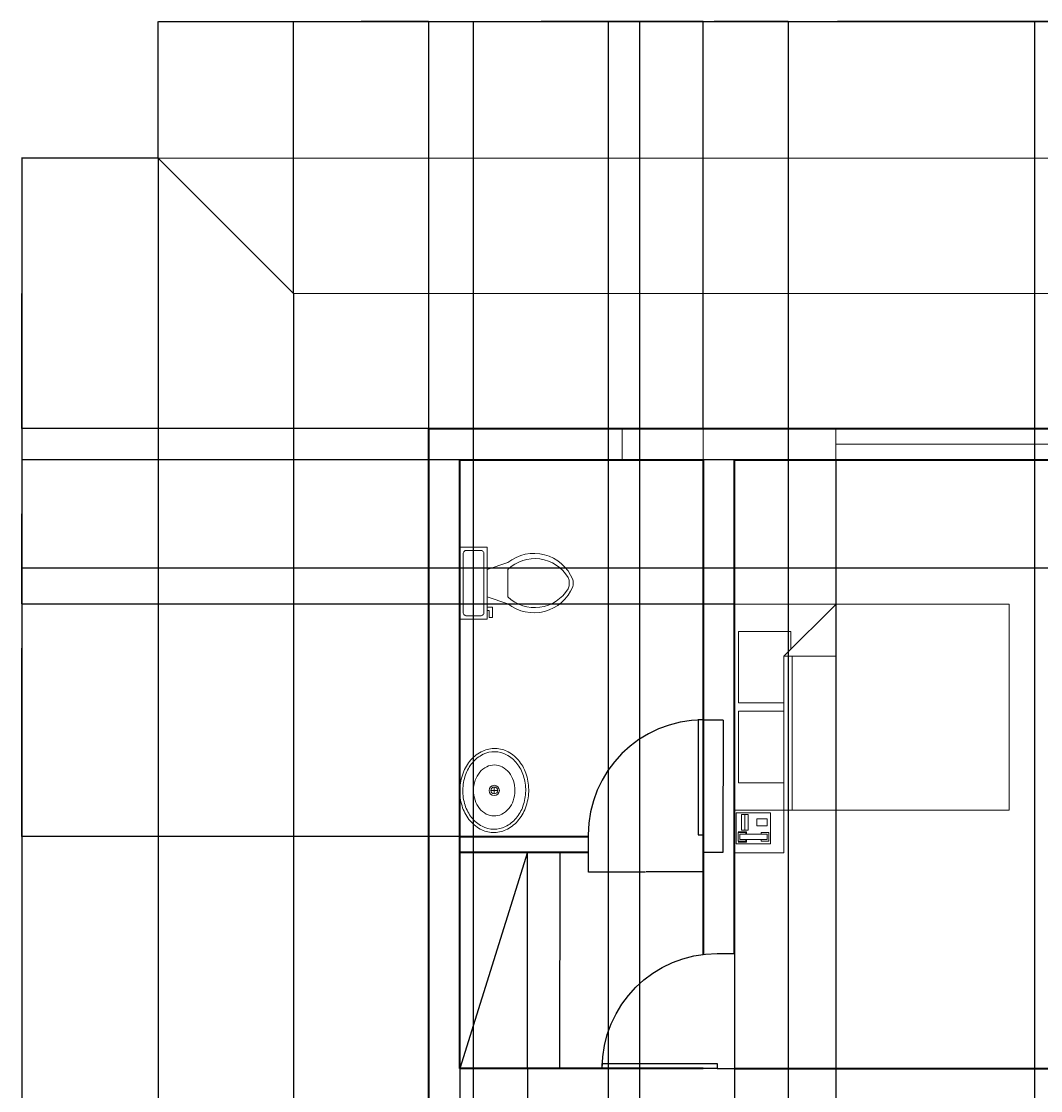
# Model space of a CAD drawing. Units: millimetres. Extents: x -8052 to 19968, y -37825 to -17505.
# Tile 6 of 10: x -8052 to -516, y -25407 to -17505. Entities that reach past the tile are written whole.
import ezdxf

# ---------------------------------------------------------------- set-up
doc = ezdxf.new("R2010")
doc.units = ezdxf.units.MM
doc.header["$MEASUREMENT"] = 0
for name, color, linetype, lineweight in [('A-ANNO-DIMS', 2, 'Continuous', 18), ('A-DOOR', 3, 'Continuous', 25), ('A-EQPM', 8, 'Continuous', 18), ('A-FLOR', 8, 'Continuous', 18), ('A-FLOR-CASE', 9, 'Continuous', 25), ('A-FLOR-FIXT', 9, 'Continuous', 18), ('A-FURN', 8, 'Continuous', 18), ('A-GLAZ', 4, 'Continuous', 18), ('A-WALL', 7, 'Continuous', 35)]:
    doc.layers.add(name, color=color, linetype=linetype, lineweight=lineweight)
doc.styles.get("Standard").update_dxf_attribs({"font": 'arial.ttf'})
doc.dimstyles.get("Standard").update_dxf_attribs({"dimtxt": 1.054, "dimasz": 1.055, "dimexe": 0.18, "dimexo": 0.0625, "dimgap": 0.09, "dimtad": 0, "dimtih": 1, "dimtoh": 1, "dimdec": 4, "dimzin": 0, "dimdsep": 46, "dimtxsty": 'Standard', "dimcen": 0.09, "dimadec": 0, "dimazin": 0, "dimtfac": 1, "dimtdec": 4, "dimtofl": 0, "dimtmove": 0, "dimatfit": 3, "dimfxl": 1, "dimtolj": 1, "dimtzin": 0, "dimarcsym": 0})

# ---------------------------------------------------------------- blocks, each defined once
blk = doc.blocks.new('Sink - Oval top')
for p, q in [((-1, 0), (1, 0)), ((0, 1), (0, -1))]:
    blk.add_line(p, q)
for points in [[(-12.23, 0.39, 0.117634), (-11.46, -3.36, 0.104469), (-8.88, -6.8, 0.090016), (-5.08, -9.07, 0.08192), (-0.32, -10.02, 0.08192), (4.49, -9.38, 0.090016), (8.42, -7.36, 0.104469), (11.22, -4.09, 0.117634), (12.23, -0.39, 0.117634), (11.46, 3.36, 0.104469), (8.88, 6.8, 0.090016), (5.08, 9.07, 0.08192), (0.32, 10.02, 0.08192), (-4.49, 9.38, 0.090016), (-8.42, 7.36, 0.104469), (-11.22, 4.09, 0.117634)], [(-11.29, 0.16, 0.118622), (-10.52, -3.25, 0.104678), (-8.07, -6.36, 0.089562), (-4.54, -8.37, 0.081185), (-0.13, -9.15, 0.081185), (4.3, -8.49, 0.089562), (7.89, -6.58, 0.104678), (10.42, -3.55, 0.118622), (11.29, -0.16, 0.118622), (10.52, 3.25, 0.104678), (8.07, 6.36, 0.089562), (4.54, 8.37, 0.081185), (0.13, 9.15, 0.081185), (-4.3, 8.49, 0.089562), (-7.89, 6.58, 0.104678), (-10.42, 3.55, 0.118622)], [(-7.42, 0.08, 0.118283), (-6.91, -2.17, 0.104607), (-5.29, -4.21, 0.089718), (-2.97, -5.53, 0.081436), (-0.07, -6.04, 0.081436), (2.84, -5.59, 0.089718), (5.2, -4.33, 0.104607), (6.86, -2.32, 0.118283), (7.42, -0.08, 0.118283), (6.91, 2.17, 0.104607), (5.29, 4.21, 0.089718), (2.97, 5.53, 0.081436), (0.07, 6.04, 0.081436), (-2.84, 5.59, 0.089718), (-5.2, 4.33, 0.104607), (-6.86, 2.32, 0.118283)]]:
    blk.add_lwpolyline(points, format="xyb", close=True)
for radius in [1.5, 1]:
    blk.add_circle((0, 0), radius)
blk = doc.blocks.new('Toilet - top')
for p, q in [((9.5, -6), (9.5, -2)), ((-10, -8.5), (-8, -8.5)), ((-10, -9.5), (-10, -8.5)), ((-8, -8.5), (-8, -8)), ((-7, -8), (-7, -9.5)), ((-4, -8), (-6, -14)), ((4, -8), (6, -14)), ((-7, -9.5), (-10, -9.5)), ((4, -14), (-4, -14))]:
    blk.add_line(p, q)
blk.add_lwpolyline([(10.5, -8), (10.5, 0), (-10.5, 0), (-10.5, -8)], close=True)
for points in [[(-9.5, -2), (-9.5, -6)], [(8.5, -1), (-8.5, -1)], [(-8.5, -7), (8.5, -7)]]:
    blk.add_lwpolyline(points)
for centre, radius, start, end in [((-8.62, -1.88), 0.884, 81.8699, 188.1301), ((8.62, -1.88), 0.884, 351.8699, 98.1301), ((-8.62, -6.12), 0.884, 171.8699, 278.1301), ((8.62, -6.12), 0.884, 261.8699, 8.1301), ((3.52, -21.58), 12.17, 141.4691, 247.9714), ((4.2, -21.82), 11.33, 136.3677, 238.9468), ((-3.52, -21.58), 12.17, 292.0284, 38.5307), ((-4.2, -21.82), 11.33, 301.053, 43.6321), ((0, -27.88), 4, 245.7318, 294.2682), ((0, -29), 4, 254.8605, 285.1395)]:
    blk.add_arc(centre, radius, start, end)
blk = doc.blocks.new('Bed - Queen')
for p, q in [((0, -80.00003), (0, 0)), ((0, 0), (59.99999, 0)), ((59.99999, 0), (59.99999, -80.00003)), ((7.99999, -1.2), (28.79998, -1.2)), ((7.99999, -14.4), (7.99999, -1.2)), ((28.79998, -1.2), (28.79998, -14.4)), ((31.19999, -1.2), (51.99999, -1.2)), ((31.19999, -14.4), (31.19999, -1.2)), ((51.99999, -1.2), (51.99999, -16.4)), ((0, -14.4), (44.8, -14.4)), ((59.99999, -29.6), (44.8, -14.4)), ((44.8, -14.4), (44.8, -29.6)), ((44.8, -16.8), (0, -16.8)), ((51.99999, -16.4), (46.79936, -16.4)), ((44.8, -29.6), (59.99999, -29.6)), ((59.99999, -80.00003), (0, -80.00003))]:
    blk.add_line(p, q)
blk = doc.blocks.new('Phone - Desk')
for p, q in [((-4.5, -5), (-4.5, 5)), ((-4.5, 5), (4.5, 5)), ((-4, 4.5), (-4, 2)), ((-3.75, 4.5), (-3.75, 2.25)), ((-1.25, 4.5), (-3.75, 4.5)), ((-3.25, 4), (-3.25, -4)), ((-3.25, 4), (-1.75, 4)), ((-1.75, -4), (-1.75, 4)), ((-1.25, 2.25), (-1.25, 4.5)), ((-1, 2), (-1, 4.5)), ((4, 3.5), (-0.5, 3.5)), ((-0.5, 3.5), (-0.5, 1.5)), ((4, 1.5), (4, 3.5)), ((4.5, 5), (4.5, -5)), ((-4, 2), (-3.25, 2)), ((-3.75, 2.25), (-3.25, 2.25)), ((-1.75, 2.25), (-1.25, 2.25)), ((-1.75, 2), (-1, 2)), ((-0.5, 2.5), (4, 2.5)), ((-0.5, 1.5), (4, 1.5)), ((-3.75, -2.25), (-3.25, -2.25)), ((-3.75, -4.5), (-3.75, -2.25)), ((-1.75, -2.25), (-1.25, -2.25)), ((-1.25, -2.25), (-1.25, -4.5)), ((2.75, -1), (0.75, -1)), ((0.75, -1), (0.75, -4)), ((2.75, -4), (2.75, -1)), ((4.5, -5), (-4.5, -5)), ((-1.25, -4.5), (-3.75, -4.5)), ((-3.25, -4), (-1.75, -4)), ((0.75, -4), (2.75, -4))]:
    blk.add_line(p, q)
blk = doc.blocks.new('TABLE-BEDSIDE')
for p, q in [((365.8, 315.3), (365.8, 0)), ((365.8, 0), (0, 0))]:
    blk.add_line(p, q)
blk = doc.blocks.new('DOOR-SWING-850')
for p, q in [((0, 127.5), (0, 0)), ((850, 127.5), (850, 0))]:
    blk.add_line(p, q)
blk.add_lwpolyline([(850, 127.5), (850, 977.5), (812.8, 977.5), (812.8, 127.5)], close=True)
blk.add_arc((850, 127.5), 850, 90, 180)
blk = doc.blocks.new('WIN-2000')
for p, q in [((0, 0), (0, 230)), ((2000, 0), (2000, 230)), ((0, 115), (2000, 115))]:
    blk.add_line(p, q)
blk = doc.blocks.new('VENT-OPENING-600')
for p, q in [((0, 0), (0, 230)), ((600, 0), (600, 230))]:
    blk.add_line(p, q)
blk = doc.blocks.new('CABINET-RECESSED-1600')
for p, q in [((500, 1600), (0, 0)), ((500, 0), (500, 1600))]:
    blk.add_line(p, q)
blk = doc.blocks.new('*D56')
at = {"layer": 'A-ANNO-DIMS', "color": 0, "lineweight": -2, "transparency": 16777216}
for p, q in [((-3010, -22667.3), (-2863.2, -22667.3)), ((-2863.4, -22668.4), (-2863.4, -23155.5)), ((-2863.4, -23643.8), (-2863.4, -23156.7)), ((-3010, -23644.8), (-2863.2, -23644.8))]:
    blk.add_line(p, q, dxfattribs=at)
at = {"layer": 'A-ANNO-DIMS', "color": 0, "lineweight": 100, "transparency": 16777216}
for points in [[(-2863.6, -22668.4), (-2863.2, -22668.4), (-2863.4, -22667.3)], [(-2863.6, -23643.8), (-2863.2, -23643.8), (-2863.4, -23644.8)]]:
    blk.add_solid(points, dxfattribs=at)
at = {"layer": 'Defpoints', "color": 0, "lineweight": 100, "transparency": 16777216}
for p in [(-3010, -22667.3), (-2863.4, -22667.3), (-3010, -23644.8)]:
    blk.add_point(p, dxfattribs=at)
at = {"layer": 'A-ANNO-DIMS', "color": 0, "transparency": 16777216, "insert": (-2863.4, -23156.1), "char_height": 1.054, "attachment_point": 5}
blk.add_mtext('\\A1;BATH DOOR 978 TYP.', dxfattribs=at)
blk = doc.blocks.new('*D57')
at = {"layer": 'A-ANNO-DIMS', "color": 0, "lineweight": -2, "transparency": 16777216}
for p, q in [((-3860, -23644.9), (-3860, -23791.6)), ((-3010, -23644.9), (-3010, -23791.6)), ((-3859, -23791.5), (-3438.1, -23791.5)), ((-3011.1, -23791.5), (-3432, -23791.5))]:
    blk.add_line(p, q, dxfattribs=at)
at = {"layer": 'A-ANNO-DIMS', "color": 0, "lineweight": 100, "transparency": 16777216}
for points in [[(-3859, -23791.3), (-3859, -23791.6), (-3860, -23791.5)], [(-3011.1, -23791.3), (-3011.1, -23791.6), (-3010, -23791.5)]]:
    blk.add_solid(points, dxfattribs=at)
at = {"layer": 'Defpoints', "color": 0, "lineweight": 100, "transparency": 16777216}
for p in [(-3860, -23644.8), (-3010, -23644.8), (-3010, -23791.5)]:
    blk.add_point(p, dxfattribs=at)
at = {"layer": 'A-ANNO-DIMS', "color": 0, "transparency": 16777216, "insert": (-3435, -23791.5), "char_height": 1.054, "attachment_point": 5}
blk.add_mtext('\\A1;850 TYP.', dxfattribs=at)
blk = doc.blocks.new('*D68')
at = {"layer": 'A-ANNO-DIMS', "color": 0, "lineweight": -2, "transparency": 16777216}
for p, q in [((-4310, -23644.8), (-4069.8, -23644.8)), ((-4070, -23645.9), (-4070, -24444.2)), ((-4070, -25243.8), (-4070, -24445.5)), ((-4310, -25244.8), (-4069.8, -25244.8))]:
    blk.add_line(p, q, dxfattribs=at)
at = {"layer": 'A-ANNO-DIMS', "color": 0, "lineweight": 100, "transparency": 16777216}
for points in [[(-4070.2, -23645.9), (-4069.8, -23645.9), (-4070, -23644.8)], [(-4070.2, -25243.8), (-4069.8, -25243.8), (-4070, -25244.8)]]:
    blk.add_solid(points, dxfattribs=at)
at = {"layer": 'Defpoints', "color": 0, "lineweight": 100, "transparency": 16777216}
for p in [(-4310, -23644.8), (-4070, -23644.8), (-4310, -25244.8)]:
    blk.add_point(p, dxfattribs=at)
at = {"layer": 'A-ANNO-DIMS', "color": 0, "transparency": 16777216, "insert": (-4070, -24444.8), "char_height": 1.054, "attachment_point": 5}
blk.add_mtext('\\A1;CABINET 1600 TYP.', dxfattribs=at)
blk = doc.blocks.new('*D69')
at = {"layer": 'A-ANNO-DIMS', "color": 0, "lineweight": -2, "transparency": 16777216}
for p, q in [((-4810, -25244.9), (-4810, -25485)), ((-4310, -25244.9), (-4310, -25485)), ((-4809, -25484.8), (-4563.1, -25484.8)), ((-4311.1, -25484.8), (-4557, -25484.8))]:
    blk.add_line(p, q, dxfattribs=at)
at = {"layer": 'A-ANNO-DIMS', "color": 0, "lineweight": 100, "transparency": 16777216}
for points in [[(-4809, -25484.7), (-4809, -25485), (-4810, -25484.8)], [(-4311.1, -25484.7), (-4311.1, -25485), (-4310, -25484.8)]]:
    blk.add_solid(points, dxfattribs=at)
at = {"layer": 'Defpoints', "color": 0, "lineweight": 100, "transparency": 16777216}
for p in [(-4810, -25244.8), (-4310, -25244.8), (-4310, -25484.8)]:
    blk.add_point(p, dxfattribs=at)
at = {"layer": 'A-ANNO-DIMS', "color": 0, "transparency": 16777216, "insert": (-4560, -25484.8), "char_height": 1.054, "attachment_point": 5}
blk.add_mtext('\\A1;500 TYP.', dxfattribs=at)
blk = doc.blocks.new('*D84')
at = {"layer": 'A-ANNO-DIMS', "color": 0, "lineweight": -2, "transparency": 16777216}
for p, q in [((-7040, -18514.8), (-7040, -17505.2)), ((-7039, -17505.3), (3022.9, -17505.3)), ((13088.9, -17505.3), (3027.1, -17505.3)), ((13090, -18514.8), (13090, -17505.2))]:
    blk.add_line(p, q, dxfattribs=at)
at = {"layer": 'A-ANNO-DIMS', "color": 0, "lineweight": 100, "transparency": 16777216}
for points in [[(-7039, -17505.2), (-7039, -17505.5), (-7040, -17505.3)], [(13088.9, -17505.2), (13088.9, -17505.5), (13090, -17505.3)]]:
    blk.add_solid(points, dxfattribs=at)
at = {"layer": 'Defpoints', "color": 0, "lineweight": 100, "transparency": 16777216}
for p in [(13090, -17505.3), (-7040, -18514.8), (13090, -18514.8)]:
    blk.add_point(p, dxfattribs=at)
at = {"layer": 'A-ANNO-DIMS', "color": 0, "transparency": 16777216, "insert": (3025, -17505.3), "char_height": 1.05, "attachment_point": 5}
blk.add_mtext('\\A1;20130', dxfattribs=at)
blk = doc.blocks.new('*D85')
at = {"layer": 'A-ANNO-DIMS', "color": 0, "lineweight": -2, "transparency": 16777216}
for p, q in [((-7040.1, -18514.8), (-8049.7, -18514.8)), ((-8049.5, -18515.9), (-8049.5, -27664.2)), ((-8049.5, -36813.8), (-8049.5, -27665.5)), ((-4710.1, -36814.8), (-8049.7, -36814.8))]:
    blk.add_line(p, q, dxfattribs=at)
at = {"layer": 'A-ANNO-DIMS', "color": 0, "lineweight": 100, "transparency": 16777216}
for points in [[(-8049.7, -18515.9), (-8049.3, -18515.9), (-8049.5, -18514.8)], [(-8049.7, -36813.8), (-8049.3, -36813.8), (-8049.5, -36814.8)]]:
    blk.add_solid(points, dxfattribs=at)
at = {"layer": 'Defpoints', "color": 0, "lineweight": 100, "transparency": 16777216}
for p in [(-7040, -18514.8), (-8049.5, -36814.8), (-4710, -36814.8)]:
    blk.add_point(p, dxfattribs=at)
at = {"layer": 'A-ANNO-DIMS', "color": 0, "transparency": 16777216, "insert": (-8049.5, -27664.8), "char_height": 1.05, "attachment_point": 5}
blk.add_mtext('\\A1;18300', dxfattribs=at)
blk = doc.blocks.new('*D86')
at = {"layer": 'A-ANNO-DIMS', "color": 0, "lineweight": -2, "transparency": 16777216}
for p, q in [((-7040, -18514.9), (-7040, -37824.5)), ((-6040, -19514.9), (-6040, -37824.5)), ((-7039, -37824.3), (-6541.6, -37824.3)), ((-6041.1, -37824.3), (-6538.4, -37824.3))]:
    blk.add_line(p, q, dxfattribs=at)
at = {"layer": 'A-ANNO-DIMS', "color": 0, "lineweight": 100, "transparency": 16777216}
for points in [[(-7039, -37824.2), (-7039, -37824.5), (-7040, -37824.3)], [(-6041.1, -37824.2), (-6041.1, -37824.5), (-6040, -37824.3)]]:
    blk.add_solid(points, dxfattribs=at)
at = {"layer": 'Defpoints', "color": 0, "lineweight": 100, "transparency": 16777216}
for p in [(-7040, -18514.8), (-6040, -19514.8), (-6040, -37824.3)]:
    blk.add_point(p, dxfattribs=at)
at = {"layer": 'A-ANNO-DIMS', "color": 0, "transparency": 16777216, "insert": (-6540, -37824.3), "char_height": 1.05, "attachment_point": 5}
blk.add_mtext('\\A1;1000', dxfattribs=at)
blk = doc.blocks.new('*D87')
at = {"layer": 'A-ANNO-DIMS', "color": 0, "lineweight": -2, "transparency": 16777216}
for p, q in [((-6040, -19514.8), (-6040, -17505.2)), ((-6039, -17505.3), (-5541.6, -17505.3)), ((-5041.1, -17505.3), (-5538.4, -17505.3)), ((-5040, -20514.8), (-5040, -17505.2))]:
    blk.add_line(p, q, dxfattribs=at)
at = {"layer": 'A-ANNO-DIMS', "color": 0, "lineweight": 100, "transparency": 16777216}
for points in [[(-6039, -17505.2), (-6039, -17505.5), (-6040, -17505.3)], [(-5041.1, -17505.2), (-5041.1, -17505.5), (-5040, -17505.3)]]:
    blk.add_solid(points, dxfattribs=at)
at = {"layer": 'Defpoints', "color": 0, "lineweight": 100, "transparency": 16777216}
for p in [(-5040, -17505.3), (-6040, -19514.8), (-5040, -20514.8)]:
    blk.add_point(p, dxfattribs=at)
at = {"layer": 'A-ANNO-DIMS', "color": 0, "transparency": 16777216, "insert": (-5540, -17505.3), "char_height": 1.05, "attachment_point": 5}
blk.add_mtext('\\A1;1000', dxfattribs=at)
blk = doc.blocks.new('*D88')
at = {"layer": 'A-ANNO-DIMS', "color": 0, "lineweight": -2, "transparency": 16777216}
for p, q in [((-7040.1, -18514.8), (-8049.7, -18514.8)), ((-8049.5, -18515.9), (-8049.5, -19514.2)), ((-8049.5, -20513.8), (-8049.5, -19515.5)), ((-5040.1, -20514.8), (-8049.7, -20514.8))]:
    blk.add_line(p, q, dxfattribs=at)
at = {"layer": 'A-ANNO-DIMS', "color": 0, "lineweight": 100, "transparency": 16777216}
for points in [[(-8049.7, -18515.9), (-8049.3, -18515.9), (-8049.5, -18514.8)], [(-8049.7, -20513.8), (-8049.3, -20513.8), (-8049.5, -20514.8)]]:
    blk.add_solid(points, dxfattribs=at)
at = {"layer": 'Defpoints', "color": 0, "lineweight": 100, "transparency": 16777216}
for p in [(-7040, -18514.8), (-8049.5, -20514.8), (-5040, -20514.8)]:
    blk.add_point(p, dxfattribs=at)
at = {"layer": 'A-ANNO-DIMS', "color": 0, "transparency": 16777216, "insert": (-8049.5, -19514.8), "char_height": 1.05, "attachment_point": 5}
blk.add_mtext('\\A1;2000', dxfattribs=at)
blk = doc.blocks.new('*D89')
at = {"layer": 'A-ANNO-DIMS', "color": 0, "lineweight": -2, "transparency": 16777216}
for p, q in [((-5040, -20514.8), (-5040, -17505.2)), ((-5039, -17505.3), (-4026.7, -17505.3)), ((-3011.1, -17505.3), (-4023.3, -17505.3)), ((-3010, -20514.8), (-3010, -17505.2))]:
    blk.add_line(p, q, dxfattribs=at)
at = {"layer": 'A-ANNO-DIMS', "color": 0, "lineweight": 100, "transparency": 16777216}
for points in [[(-5039, -17505.2), (-5039, -17505.5), (-5040, -17505.3)], [(-3011.1, -17505.2), (-3011.1, -17505.5), (-3010, -17505.3)]]:
    blk.add_solid(points, dxfattribs=at)
at = {"layer": 'Defpoints', "color": 0, "lineweight": 100, "transparency": 16777216}
for p in [(-3010, -17505.3), (-5040, -20514.8), (-3010, -20514.8)]:
    blk.add_point(p, dxfattribs=at)
at = {"layer": 'A-ANNO-DIMS', "color": 0, "transparency": 16777216, "insert": (-4025, -17505.3), "char_height": 1.05, "attachment_point": 5}
blk.add_mtext('\\A1;2030', dxfattribs=at)
blk = doc.blocks.new('*D90')
at = {"layer": 'A-ANNO-DIMS', "color": 0, "lineweight": -2, "transparency": 16777216}
for p, q in [((-3010, -20514.8), (-3010, -17505.2)), ((-3009, -17505.3), (-1146.7, -17505.3)), ((718.9, -17505.3), (-1143.4, -17505.3)), ((720, -20514.8), (720, -17505.2))]:
    blk.add_line(p, q, dxfattribs=at)
at = {"layer": 'A-ANNO-DIMS', "color": 0, "lineweight": 100, "transparency": 16777216}
for points in [[(-3009, -17505.2), (-3009, -17505.5), (-3010, -17505.3)], [(718.9, -17505.2), (718.9, -17505.5), (720, -17505.3)]]:
    blk.add_solid(points, dxfattribs=at)
at = {"layer": 'Defpoints', "color": 0, "lineweight": 100, "transparency": 16777216}
for p in [(720, -17505.3), (-3010, -20514.8), (720, -20514.8)]:
    blk.add_point(p, dxfattribs=at)
at = {"layer": 'A-ANNO-DIMS', "color": 0, "transparency": 16777216, "insert": (-1145, -17505.3), "char_height": 1.05, "attachment_point": 5}
blk.add_mtext('\\A1;3730', dxfattribs=at)
blk = doc.blocks.new('*D94')
at = {"layer": 'A-ANNO-DIMS', "color": 0, "lineweight": -2, "transparency": 16777216}
for p, q in [((-2780, -20744.9), (-2780, -37824.5)), ((-2030, -20744.9), (-2030, -37824.5)), ((-2779, -37824.3), (-2406.3, -37824.3)), ((-2031.1, -37824.3), (-2403.8, -37824.3))]:
    blk.add_line(p, q, dxfattribs=at)
at = {"layer": 'A-ANNO-DIMS', "color": 0, "lineweight": 100, "transparency": 16777216}
for points in [[(-2779, -37824.2), (-2779, -37824.5), (-2780, -37824.3)], [(-2031.1, -37824.2), (-2031.1, -37824.5), (-2030, -37824.3)]]:
    blk.add_solid(points, dxfattribs=at)
at = {"layer": 'Defpoints', "color": 0, "lineweight": 100, "transparency": 16777216}
for p in [(-2780, -20744.8), (-2030, -20744.8), (-2030, -37824.3)]:
    blk.add_point(p, dxfattribs=at)
at = {"layer": 'A-ANNO-DIMS', "color": 0, "transparency": 16777216, "insert": (-2405, -37824.3), "char_height": 1.05, "attachment_point": 5}
blk.add_mtext('\\A1;750', dxfattribs=at)
blk = doc.blocks.new('*D99')
at = {"layer": 'A-ANNO-DIMS', "color": 0, "lineweight": -2, "transparency": 16777216}
for p, q in [((-4710, -36814.8), (-4710, -17505.2)), ((-4709, -17505.3), (-4211.6, -17505.3)), ((-3711.1, -17505.3), (-4208.4, -17505.3)), ((-3710, -35814.8), (-3710, -17505.2))]:
    blk.add_line(p, q, dxfattribs=at)
at = {"layer": 'A-ANNO-DIMS', "color": 0, "lineweight": 100, "transparency": 16777216}
for points in [[(-4709, -17505.2), (-4709, -17505.5), (-4710, -17505.3)], [(-3711.1, -17505.2), (-3711.1, -17505.5), (-3710, -17505.3)]]:
    blk.add_solid(points, dxfattribs=at)
at = {"layer": 'Defpoints', "color": 0, "lineweight": 100, "transparency": 16777216}
for p in [(-3710, -17505.3), (-3710, -35814.8), (-4710, -36814.8)]:
    blk.add_point(p, dxfattribs=at)
at = {"layer": 'A-ANNO-DIMS', "color": 0, "transparency": 16777216, "insert": (-4210, -17505.3), "char_height": 1.05, "attachment_point": 5}
blk.add_mtext('\\A1;1000', dxfattribs=at)
blk = doc.blocks.new('*D103')
at = {"layer": 'A-ANNO-DIMS', "color": 0, "lineweight": -2, "transparency": 16777216}
for p, q in [((-3480, -35584.8), (-3480, -17505.2)), ((-3479, -17505.3), (-2931.6, -17505.3)), ((-2381.1, -17505.3), (-2928.4, -17505.3)), ((-2380, -35584.8), (-2380, -17505.2))]:
    blk.add_line(p, q, dxfattribs=at)
at = {"layer": 'A-ANNO-DIMS', "color": 0, "lineweight": 100, "transparency": 16777216}
for points in [[(-3479, -17505.2), (-3479, -17505.5), (-3480, -17505.3)], [(-2381.1, -17505.2), (-2381.1, -17505.5), (-2380, -17505.3)]]:
    blk.add_solid(points, dxfattribs=at)
at = {"layer": 'Defpoints', "color": 0, "lineweight": 100, "transparency": 16777216}
for p in [(-2380, -17505.3), (-3480, -35584.8), (-2380, -35584.8)]:
    blk.add_point(p, dxfattribs=at)
at = {"layer": 'A-ANNO-DIMS', "color": 0, "transparency": 16777216, "insert": (-2930, -17505.3), "char_height": 1.05, "attachment_point": 5}
blk.add_mtext('\\A1;1100', dxfattribs=at)
blk = doc.blocks.new('*D105')
at = {"layer": 'A-ANNO-DIMS', "color": 0, "lineweight": -2, "transparency": 16777216}
for p, q in [((-4810.1, -20744.8), (-8049.7, -20744.8)), ((-8049.5, -20745.9), (-8049.5, -22136.7)), ((-8049.5, -23528.8), (-8049.5, -22138)), ((-4810.1, -23529.8), (-8049.7, -23529.8))]:
    blk.add_line(p, q, dxfattribs=at)
at = {"layer": 'A-ANNO-DIMS', "color": 0, "lineweight": 100, "transparency": 16777216}
for points in [[(-8049.7, -20745.9), (-8049.3, -20745.9), (-8049.5, -20744.8)], [(-8049.7, -23528.8), (-8049.3, -23528.8), (-8049.5, -23529.8)]]:
    blk.add_solid(points, dxfattribs=at)
at = {"layer": 'Defpoints', "color": 0, "lineweight": 100, "transparency": 16777216}
for p in [(-4810, -20744.8), (-8049.5, -23529.8), (-4810, -23529.8)]:
    blk.add_point(p, dxfattribs=at)
at = {"layer": 'A-ANNO-DIMS', "color": 0, "transparency": 16777216, "insert": (-8049.5, -22137.3), "char_height": 1.05, "attachment_point": 5}
blk.add_mtext('\\A1;2785', dxfattribs=at)
blk = doc.blocks.new('*D107')
at = {"layer": 'A-ANNO-DIMS', "color": 0, "lineweight": -2, "transparency": 16777216}
for p, q in [((-3480, -30204.8), (-3480, -17505.2)), ((-3479, -17505.3), (-2021.1, -17505.3)), ((-558.6, -17505.3), (-2016.5, -17505.3)), ((-557.5, -30204.8), (-557.5, -17505.2))]:
    blk.add_line(p, q, dxfattribs=at)
at = {"layer": 'A-ANNO-DIMS', "color": 0, "lineweight": 100, "transparency": 16777216}
for points in [[(-3479, -17505.2), (-3479, -17505.5), (-3480, -17505.3)], [(-558.6, -17505.2), (-558.6, -17505.5), (-557.5, -17505.3)]]:
    blk.add_solid(points, dxfattribs=at)
at = {"layer": 'Defpoints', "color": 0, "lineweight": 100, "transparency": 16777216}
for p in [(-557.5, -17505.3), (-3480, -30204.8), (-557.5, -30204.8)]:
    blk.add_point(p, dxfattribs=at)
at = {"layer": 'A-ANNO-DIMS', "color": 0, "transparency": 16777216, "insert": (-2018.8, -17505.3), "char_height": 1.05, "attachment_point": 5}
blk.add_mtext('\\A1;2922.5', dxfattribs=at)
blk = doc.blocks.new('*D114')
at = {"layer": 'A-ANNO-DIMS', "color": 0, "lineweight": -2, "transparency": 16777216}
for p, q in [((2999.9, -20744.8), (-8049.7, -20744.8)), ((-8049.5, -20745.9), (-8049.5, -21144.2)), ((-8049.5, -21543.8), (-8049.5, -21145.5)), ((2999.9, -21544.8), (-8049.7, -21544.8))]:
    blk.add_line(p, q, dxfattribs=at)
at = {"layer": 'A-ANNO-DIMS', "color": 0, "lineweight": 100, "transparency": 16777216}
for points in [[(-8049.7, -20745.9), (-8049.3, -20745.9), (-8049.5, -20744.8)], [(-8049.7, -21543.8), (-8049.3, -21543.8), (-8049.5, -21544.8)]]:
    blk.add_solid(points, dxfattribs=at)
at = {"layer": 'Defpoints', "color": 0, "lineweight": 100, "transparency": 16777216}
for p in [(3000, -20744.8), (-8049.5, -21544.8), (3000, -21544.8)]:
    blk.add_point(p, dxfattribs=at)
at = {"layer": 'A-ANNO-DIMS', "color": 0, "transparency": 16777216, "insert": (-8049.5, -21144.8), "char_height": 1.05, "attachment_point": 5}
blk.add_mtext('\\A1;800', dxfattribs=at)
blk = doc.blocks.new('*D116')
at = {"layer": 'A-ANNO-DIMS', "color": 0, "lineweight": -2, "transparency": 16777216}
for p, q in [((-2780.1, -20744.8), (-8049.7, -20744.8)), ((-8049.5, -20745.9), (-8049.5, -21277.3)), ((-8049.5, -21809.9), (-8049.5, -21278.5)), ((-2780.1, -21810.9), (-8049.7, -21810.9))]:
    blk.add_line(p, q, dxfattribs=at)
at = {"layer": 'A-ANNO-DIMS', "color": 0, "lineweight": 100, "transparency": 16777216}
for points in [[(-8049.7, -20745.9), (-8049.3, -20745.9), (-8049.5, -20744.8)], [(-8049.7, -21809.9), (-8049.3, -21809.9), (-8049.5, -21810.9)]]:
    blk.add_solid(points, dxfattribs=at)
at = {"layer": 'Defpoints', "color": 0, "lineweight": 100, "transparency": 16777216}
for p in [(-2780, -20744.8), (-8049.5, -21810.9), (-2780, -21810.9)]:
    blk.add_point(p, dxfattribs=at)
at = {"layer": 'A-ANNO-DIMS', "color": 0, "transparency": 16777216, "insert": (-8049.5, -21277.9), "char_height": 1.05, "attachment_point": 5}
blk.add_mtext('\\A1;1066', dxfattribs=at)

msp = doc.modelspace()

# ---------------------------------------------------------------- linework, layer by layer
at = {"layer": 'A-FLOR'}
for p, q in [((-7040.021, -18514.843), (-6040.021, -19514.843)), ((-7040.021, -20744.843), (-7040.021, -18514.843)), ((-7040.021, -18514.843), (-4810.021, -18514.843)), ((-4810.021, -18514.843), (13089.979, -18514.843)), ((-6040.021, -25244.843), (-6040.021, -19514.843)), ((-6040.021, -19514.843), (12089.979, -19514.843)), ((-7040.021, -26474.843), (-7040.021, -20744.843)), ((-6040.021, -25474.843), (-6040.021, -25244.843))]:
    msp.add_line(p, q, dxfattribs=at)
at = {"layer": 'A-WALL'}
for p, q in [((-5040.021, -20514.843), (-4810.021, -20514.843)), ((-5040.021, -20744.843), (-5040.021, -20514.843)), ((-4810.021, -20514.843), (-3010.021, -20514.843)), ((-3010.021, -20514.843), (-2780.021, -20514.843)), ((-2780.021, -20514.843), (719.979, -20514.843)), ((-5040.021, -25244.843), (-5040.021, -20744.843)), ((-4810.021, -25244.843), (-4810.021, -20744.843)), ((-4810.021, -20744.843), (-3010.021, -20744.843)), ((-3010.021, -20744.843), (-3010.021, -24401.046)), ((-2780.021, -20744.843), (719.979, -20744.843)), ((-2780.021, -24394.843), (-2780.021, -20744.843)), ((-4810.021, -23529.843), (-3860.021, -23529.843)), ((-4810.021, -23644.843), (-3860.021, -23644.843)), ((-5040.021, -25474.843), (-5040.021, -25244.843)), ((-3010.021, -25244.843), (-4810.021, -25244.843)), ((-2780.021, -25244.843), (-330.021, -25244.843))]:
    msp.add_line(p, q, dxfattribs=at)

# ---------------------------------------------------------------- block references
at = {"layer": 'A-DOOR'}
msp.add_blockref('DOOR-SWING-850', (-3860.021, -23644.843), dxfattribs=at)
at = {"layer": 'A-DOOR', "extrusion": (0, 0, -1), "zscale": -1, "rotation": 270}
msp.add_blockref('DOOR-SWING-850', (2780.021, -24394.843), dxfattribs=at)
at = {"layer": 'A-EQPM', "xscale": 25.4, "yscale": 25.4, "zscale": 25.4, "rotation": 90}
msp.add_blockref('Phone - Desk', (-2638.76, -23468.572), dxfattribs=at)
at = {"layer": 'A-FLOR-CASE'}
msp.add_blockref('CABINET-RECESSED-1600', (-4810.021, -25244.843), dxfattribs=at)
at = {"layer": 'A-FLOR-FIXT', "xscale": 25.4, "yscale": 25.4, "zscale": 25.4}
for name, p, rotation in [('Toilet - top', (-4810.021, -21656.461), 90), ('Sink - Oval top', (-4555.422, -23189.112), 270)]:
    msp.add_blockref(name, p, dxfattribs=dict(at, rotation=rotation))
at = {"layer": 'A-FURN', "xscale": 25.4, "yscale": 25.4, "zscale": 25.4, "rotation": 90}
msp.add_blockref('Bed - Queen', (-2780.021, -23334.944), dxfattribs=at)
at = {"layer": 'A-FURN'}
msp.add_blockref('TABLE-BEDSIDE', (-2780.021, -23650.203), dxfattribs=at)
at = {"layer": 'A-GLAZ'}
for name, p in [('VENT-OPENING-600', (-3610.021, -20744.843)), ('WIN-2000', (-2030.021, -20744.843))]:
    msp.add_blockref(name, p, dxfattribs=at)

# ---------------------------------------------------------------- dimensions: what is measured, and where the dimension line sits
at = {"layer": 'A-ANNO-DIMS'}
for base, p1, p2, override, picture, middle in [((13089.979, -17505.343), (-7040.021, -18514.843), (13089.979, -18514.843), {"dimdec": 0, "dimlfac": 1, "dimrnd": 0, "dimzin": 0, "dimdsep": 46, "dimlunit": 2}, '*D84', (3024.979, -17505.343)), ((-5040.021, -17505.343), (-6040.021, -19514.843), (-5040.021, -20514.843), {"dimdec": 0, "dimlfac": 1, "dimrnd": 0, "dimzin": 0, "dimdsep": 46, "dimlunit": 2}, '*D87', (-5540.021, -17505.343)), ((-3010.021, -17505.343), (-5040.021, -20514.843), (-3010.021, -20514.843), {"dimdec": 0, "dimlfac": 1, "dimrnd": 0, "dimzin": 0, "dimdsep": 46, "dimlunit": 2}, '*D89', (-4025.021, -17505.343)), ((-3710.021, -17505.343), (-4710.021, -36814.843), (-3710.021, -35814.843), {"dimdec": 0, "dimlfac": 1, "dimrnd": 0, "dimzin": 0, "dimdsep": 46, "dimlunit": 2}, '*D99', (-4210.021, -17505.343)), ((-2380.021, -17505.343), (-3480.021, -35584.843), (-2380.021, -35584.843), {"dimdec": 0, "dimlfac": 1, "dimrnd": 0, "dimzin": 0, "dimdsep": 46, "dimlunit": 2}, '*D103', (-2930.021, -17505.343)), ((-557.515, -17505.343), (-3480.021, -30204.843), (-557.515, -30204.843), {"dimdec": 1, "dimlfac": 1, "dimrnd": 0, "dimzin": 0, "dimdsep": 46, "dimlunit": 2}, '*D107', (-2018.768, -17505.343)), ((719.979, -17505.343), (-3010.021, -20514.843), (719.979, -20514.843), {"dimdec": 0, "dimlfac": 1, "dimrnd": 0, "dimzin": 0, "dimdsep": 46, "dimlunit": 2}, '*D90', (-1145.021, -17505.343)), ((-6040.021, -37824.343), (-7040.021, -18514.843), (-6040.021, -19514.843), {"dimdec": 0, "dimlfac": 1, "dimrnd": 0, "dimzin": 0, "dimdsep": 46, "dimlunit": 2}, '*D86', (-6540.021, -37824.343)), ((-2030.021, -37824.343), (-2780.021, -20744.843), (-2030.021, -20744.843), {"dimdec": 0, "dimlfac": 1, "dimrnd": 0, "dimzin": 0, "dimdsep": 46, "dimlunit": 2}, '*D94', (-2405.021, -37824.343))]:
    dim = msp.add_linear_dim(base=base, p1=p1, p2=p2, dimstyle='Standard', override=override, dxfattribs=at)
    dim.commit()
    dim.dimension.update_dxf_attribs({"geometry": picture, "text_midpoint": middle})
for base, p1, p2, picture, middle in [((-8049.521, -36814.843), (-7040.021, -18514.843), (-4710.021, -36814.843), '*D85', (-8049.521, -27664.843)), ((-8049.521, -20514.843), (-7040.021, -18514.843), (-5040.021, -20514.843), '*D88', (-8049.521, -19514.843)), ((-8049.521, -23529.843), (-4810.021, -20744.843), (-4810.021, -23529.843), '*D105', (-8049.521, -22137.343)), ((-8049.521, -21810.945), (-2780.021, -20744.843), (-2780.021, -21810.945), '*D116', (-8049.521, -21277.894)), ((-8049.521, -21544.843), (2999.979, -20744.843), (2999.979, -21544.843), '*D114', (-8049.521, -21144.843))]:
    dim = msp.add_linear_dim(base=base, p1=p1, p2=p2, angle=90, dimstyle='Standard', override={"dimdec": 0, "dimlfac": 1, "dimrnd": 0, "dimzin": 0, "dimdsep": 46, "dimlunit": 2}, dxfattribs=at)
    dim.commit()
    dim.dimension.update_dxf_attribs({"geometry": picture, "text_midpoint": middle})
for base, p1, p2, text, picture, middle in [((-2863.395628322, -22667.34303639), (-3010.020628322, -23644.84303639), (-3010.020628322, -22667.34303639), 'BATH DOOR <> TYP.', '*D56', (-2863.395628322, -23156.09303639)), ((-4070.021, -23644.843), (-4310.021, -25244.843), (-4310.021, -23644.843), 'CABINET <> TYP.', '*D68', (-4070.021, -24444.843))]:
    dim = msp.add_linear_dim(base=base, p1=p1, p2=p2, angle=90, text=text, dimstyle='Standard', override={"dimdec": 0, "dimlfac": 1, "dimrnd": 0, "dimzin": 0, "dimdsep": 46, "dimlunit": 2}, dxfattribs=at)
    dim.commit()
    dim.dimension.update_dxf_attribs({"geometry": picture, "text_midpoint": middle})
for base, p1, p2, picture, middle in [((-3010.021, -23791.468), (-3860.021, -23644.843), (-3010.021, -23644.843), '*D57', (-3435.021, -23791.468)), ((-4310.021, -25484.843), (-4810.021, -25244.843), (-4310.021, -25244.843), '*D69', (-4560.021, -25484.843))]:
    dim = msp.add_linear_dim(base=base, p1=p1, p2=p2, text='<> TYP.', dimstyle='Standard', override={"dimdec": 0, "dimlfac": 1, "dimrnd": 0, "dimzin": 0, "dimdsep": 46, "dimlunit": 2}, dxfattribs=at)
    dim.commit()
    dim.dimension.update_dxf_attribs({"geometry": picture, "text_midpoint": middle})

doc.saveas('drawing.dxf')
